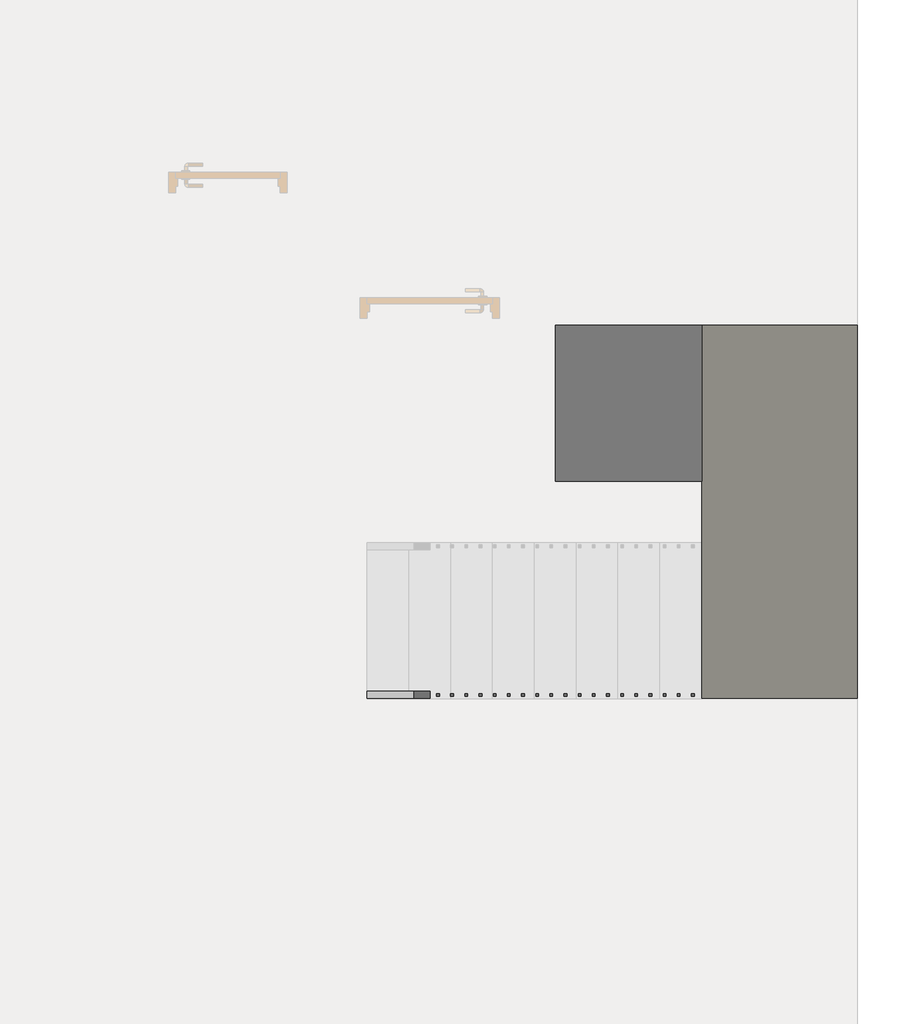
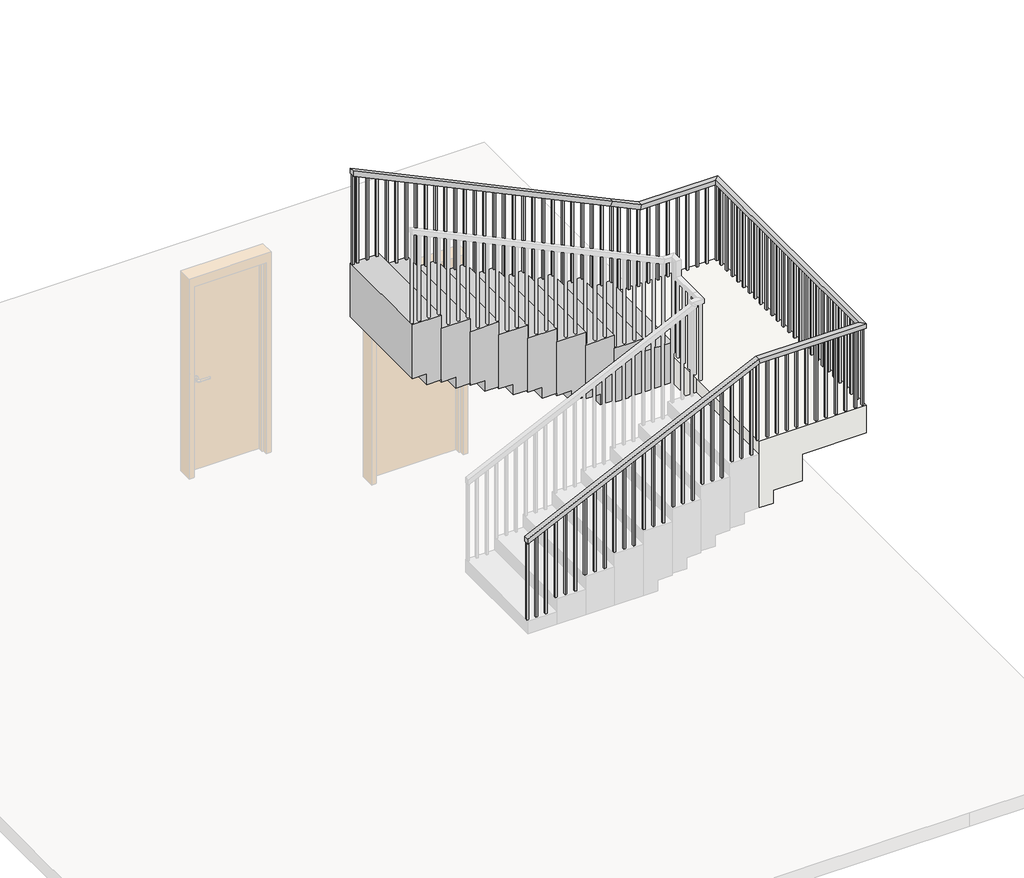
# One storey, part 2 of 2: 1 railing, 1 slab, 1 stair flight.
"""IFC4 building model written with IfcOpenShell, lengths in millimetres."""

from ifc_helpers import new_model, si_unit, frame, origin, place, context, project, spatial, polyline, outline, extrude, faceted_brep, element, save

model = new_model("IFC4")

# Units and contexts
model_context = context("Model", 3, world=origin())
ifc_project = project(units=[si_unit("LENGTHUNIT", "METRE", prefix="MILLI")], contexts=[model_context])

# Site, building, storey
site = spatial("IfcSite", under=ifc_project)
building = spatial("IfcBuilding", under=site)
storey = spatial("IfcBuildingStorey", under=building, Elevation=600.0)

# Railing
placement = place(None, origin())
element("IfcRailing", 1, ObjectType="Handrail - Rectangular", at=placement, inside=storey, context=model_context, shape_type="SolidModel", body=[
    faceted_brep([(-11513.3520625, -4858.6480844, 1642.1052632), (-11513.3520625, -4858.6480844, 1586.7794841), (-11513.3520625, -4908.6480844, 1586.7794841), (-11513.3520625, -4908.6480844, 1642.1052632), (-9113.3520625, -4858.6480844, 2778.9473684), (-9102.1087512, -4858.6480844, 2728.9473684), (-9102.1087512, -4908.6480844, 2728.9473684), (-9113.3520625, -4908.6480844, 2778.9473684), (-8046.1520625, -4858.6480844, 2778.9473684), (-8046.1520625, -4858.6480844, 2728.9473684), (-7996.1520625, -4908.6480844, 2728.9473684), (-7996.1520625, -4908.6480844, 2778.9473684), (-8046.1520625, -2284.4480844, 2778.9473684), (-8046.1520625, -2284.4480844, 2728.9473684), (-7996.1520625, -2234.4480844, 2728.9473684), (-7996.1520625, -2234.4480844, 2778.9473684), (-8813.3520625, -2284.4480844, 2778.9473684), (-8824.5953738, -2284.4480844, 2728.9473684), (-8824.5953738, -2234.4480844, 2728.9473684), (-8813.3520625, -2234.4480844, 2778.9473684), (-9113.3520625, -2284.4480844, 2921.0526316), (-9134.7563797, -2284.4480844, 2875.8657396), (-9134.7563797, -2234.4480844, 2875.8657396), (-9113.3520625, -2234.4480844, 2921.0526316), (-11813.3520625, -2284.4480844, 4200.0), (-11813.3520625, -2234.4480844, 4200.0), (-11813.3520625, -2234.4480844, 4144.6742209), (-11813.3520625, -2284.4480844, 4144.6742209)], [[[0, 1, 2, 3]], [[1, 0, 4, 5]], [[2, 1, 5, 6]], [[3, 2, 6, 7]], [[0, 3, 7, 4]], [[5, 4, 8, 9]], [[6, 5, 9, 10]], [[7, 6, 10, 11]], [[4, 7, 11, 8]], [[9, 8, 12, 13]], [[10, 9, 13, 14]], [[11, 10, 14, 15]], [[8, 11, 15, 12]], [[13, 12, 16, 17]], [[14, 13, 17, 18]], [[15, 14, 18, 19]], [[12, 15, 19, 16]], [[17, 16, 20, 21]], [[18, 17, 21, 22]], [[19, 18, 22, 23]], [[16, 19, 23, 20]], [[24, 25, 26, 27]], [[21, 20, 24, 27]], [[22, 21, 27, 26]], [[23, 22, 26, 25]], [[20, 23, 25, 24]]]),
    extrude(outline(polyline([(3157.8947368, -11744.9520625), (4112.2742209, -11744.9520625), (4121.7479052, -11764.9520625), (3157.8947368, -11764.9520625), (3157.8947368, -11744.9520625)])), frame((0.0, -2269.4480844, 0.0), z_axis=(0.0, 1.0, 0.0), x_axis=(0.0, 0.0, 1.0)), (0.0, 0.0, 1.0), 20.0),
    extrude(outline(polyline([(3157.8947368, -11643.3520625), (4064.1479052, -11643.3520625), (4073.6215894, -11663.3520625), (3157.8947368, -11663.3520625), (3157.8947368, -11643.3520625)])), frame((0.0, -2269.4480844, 0.0), z_axis=(0.0, 1.0, 0.0), x_axis=(0.0, 0.0, 1.0)), (0.0, 0.0, 1.0), 20.0),
    extrude(outline(polyline([(3157.8947368, -11541.7520625), (4016.0215894, -11541.7520625), (4025.4952736, -11561.7520625), (3157.8947368, -11561.7520625), (3157.8947368, -11541.7520625)])), frame((0.0, -2269.4480844, 0.0), z_axis=(0.0, 1.0, 0.0), x_axis=(0.0, 0.0, 1.0)), (0.0, 0.0, 1.0), 20.0),
    extrude(outline(polyline([(3015.7894737, -11440.1520625), (3967.8952736, -11440.1520625), (3977.3689578, -11460.1520625), (3015.7894737, -11460.1520625), (3015.7894737, -11440.1520625)])), frame((0.0, -2269.4480844, 0.0), z_axis=(0.0, 1.0, 0.0), x_axis=(0.0, 0.0, 1.0)), (0.0, 0.0, 1.0), 20.0),
    extrude(outline(polyline([(3015.7894737, -11338.5520625), (3919.7689578, -11338.5520625), (3929.242642, -11358.5520625), (3015.7894737, -11358.5520625), (3015.7894737, -11338.5520625)])), frame((0.0, -2269.4480844, 0.0), z_axis=(0.0, 1.0, 0.0), x_axis=(0.0, 0.0, 1.0)), (0.0, 0.0, 1.0), 20.0),
    extrude(outline(polyline([(3015.7894737, -11236.9520625), (3871.642642, -11236.9520625), (3881.1163262, -11256.9520625), (3015.7894737, -11256.9520625), (3015.7894737, -11236.9520625)])), frame((0.0, -2269.4480844, 0.0), z_axis=(0.0, 1.0, 0.0), x_axis=(0.0, 0.0, 1.0)), (0.0, 0.0, 1.0), 20.0),
    extrude(outline(polyline([(2873.6842105, -11135.3520625), (3823.5163262, -11135.3520625), (3832.9900104, -11155.3520625), (2873.6842105, -11155.3520625), (2873.6842105, -11135.3520625)])), frame((0.0, -2269.4480844, 0.0), z_axis=(0.0, 1.0, 0.0), x_axis=(0.0, 0.0, 1.0)), (0.0, 0.0, 1.0), 20.0),
    extrude(outline(polyline([(2873.6842105, -11033.7520625), (3775.3900104, -11033.7520625), (3784.8636946, -11053.7520625), (2873.6842105, -11053.7520625), (2873.6842105, -11033.7520625)])), frame((0.0, -2269.4480844, 0.0), z_axis=(0.0, 1.0, 0.0), x_axis=(0.0, 0.0, 1.0)), (0.0, 0.0, 1.0), 20.0),
    extrude(outline(polyline([(2873.6842105, -10932.1520625), (3727.2636946, -10932.1520625), (3736.7373788, -10952.1520625), (2873.6842105, -10952.1520625), (2873.6842105, -10932.1520625)])), frame((0.0, -2269.4480844, 0.0), z_axis=(0.0, 1.0, 0.0), x_axis=(0.0, 0.0, 1.0)), (0.0, 0.0, 1.0), 20.0),
    extrude(outline(polyline([(2731.5789474, -10830.5520625), (3679.1373788, -10830.5520625), (3688.611063, -10850.5520625), (2731.5789474, -10850.5520625), (2731.5789474, -10830.5520625)])), frame((0.0, -2269.4480844, 0.0), z_axis=(0.0, 1.0, 0.0), x_axis=(0.0, 0.0, 1.0)), (0.0, 0.0, 1.0), 20.0),
    extrude(outline(polyline([(2731.5789474, -10728.9520625), (3631.011063, -10728.9520625), (3640.4847473, -10748.9520625), (2731.5789474, -10748.9520625), (2731.5789474, -10728.9520625)])), frame((0.0, -2269.4480844, 0.0), z_axis=(0.0, 1.0, 0.0), x_axis=(0.0, 0.0, 1.0)), (0.0, 0.0, 1.0), 20.0),
    extrude(outline(polyline([(2731.5789474, -10627.3520625), (3582.8847473, -10627.3520625), (3592.3584315, -10647.3520625), (2731.5789474, -10647.3520625), (2731.5789474, -10627.3520625)])), frame((0.0, -2269.4480844, 0.0), z_axis=(0.0, 1.0, 0.0), x_axis=(0.0, 0.0, 1.0)), (0.0, 0.0, 1.0), 20.0),
    extrude(outline(polyline([(2589.4736842, -10525.7520625), (3534.7584315, -10525.7520625), (3544.2321157, -10545.7520625), (2589.4736842, -10545.7520625), (2589.4736842, -10525.7520625)])), frame((0.0, -2269.4480844, 0.0), z_axis=(0.0, 1.0, 0.0), x_axis=(0.0, 0.0, 1.0)), (0.0, 0.0, 1.0), 20.0),
    extrude(outline(polyline([(2589.4736842, -10424.1520625), (3486.6321157, -10424.1520625), (3496.1057999, -10444.1520625), (2589.4736842, -10444.1520625), (2589.4736842, -10424.1520625)])), frame((0.0, -2269.4480844, 0.0), z_axis=(0.0, 1.0, 0.0), x_axis=(0.0, 0.0, 1.0)), (0.0, 0.0, 1.0), 20.0),
    extrude(outline(polyline([(2589.4736842, -10322.5520625), (3438.5057999, -10322.5520625), (3447.9794841, -10342.5520625), (2589.4736842, -10342.5520625), (2589.4736842, -10322.5520625)])), frame((0.0, -2269.4480844, 0.0), z_axis=(0.0, 1.0, 0.0), x_axis=(0.0, 0.0, 1.0)), (0.0, 0.0, 1.0), 20.0),
    extrude(outline(polyline([(2447.3684211, -10220.9520625), (3390.3794841, -10220.9520625), (3399.8531683, -10240.9520625), (2447.3684211, -10240.9520625), (2447.3684211, -10220.9520625)])), frame((0.0, -2269.4480844, 0.0), z_axis=(0.0, 1.0, 0.0), x_axis=(0.0, 0.0, 1.0)), (0.0, 0.0, 1.0), 20.0),
    extrude(outline(polyline([(2447.3684211, -10119.3520625), (3342.2531683, -10119.3520625), (3351.7268525, -10139.3520625), (2447.3684211, -10139.3520625), (2447.3684211, -10119.3520625)])), frame((0.0, -2269.4480844, 0.0), z_axis=(0.0, 1.0, 0.0), x_axis=(0.0, 0.0, 1.0)), (0.0, 0.0, 1.0), 20.0),
    extrude(outline(polyline([(2447.3684211, -10017.7520625), (3294.1268525, -10017.7520625), (3303.6005367, -10037.7520625), (2447.3684211, -10037.7520625), (2447.3684211, -10017.7520625)])), frame((0.0, -2269.4480844, 0.0), z_axis=(0.0, 1.0, 0.0), x_axis=(0.0, 0.0, 1.0)), (0.0, 0.0, 1.0), 20.0),
    extrude(outline(polyline([(2305.2631579, -9916.1520625), (3246.0005367, -9916.1520625), (3255.4742209, -9936.1520625), (2305.2631579, -9936.1520625), (2305.2631579, -9916.1520625)])), frame((0.0, -2269.4480844, 0.0), z_axis=(0.0, 1.0, 0.0), x_axis=(0.0, 0.0, 1.0)), (0.0, 0.0, 1.0), 20.0),
    extrude(outline(polyline([(2305.2631579, -9814.5520625), (3197.8742209, -9814.5520625), (3207.3479052, -9834.5520625), (2305.2631579, -9834.5520625), (2305.2631579, -9814.5520625)])), frame((0.0, -2269.4480844, 0.0), z_axis=(0.0, 1.0, 0.0), x_axis=(0.0, 0.0, 1.0)), (0.0, 0.0, 1.0), 20.0),
    extrude(outline(polyline([(2305.2631579, -9712.9520625), (3149.7005367, -9712.9520625), (3159.1742209, -9732.9520625), (2305.2631579, -9732.9520625), (2305.2631579, -9712.9520625)])), frame((0.0, -2269.4480844, 0.0), z_axis=(0.0, 1.0, 0.0), x_axis=(0.0, 0.0, 1.0)), (0.0, 0.0, 1.0), 20.0),
    extrude(outline(polyline([(2163.1578947, -9611.3520625), (3101.6215894, -9611.3520625), (3111.0952736, -9631.3520625), (2163.1578947, -9631.3520625), (2163.1578947, -9611.3520625)])), frame((0.0, -2269.4480844, 0.0), z_axis=(0.0, 1.0, 0.0), x_axis=(0.0, 0.0, 1.0)), (0.0, 0.0, 1.0), 20.0),
    extrude(outline(polyline([(2163.1578947, -9509.7520625), (3053.4952736, -9509.7520625), (3062.9689578, -9529.7520625), (2163.1578947, -9529.7520625), (2163.1578947, -9509.7520625)])), frame((0.0, -2269.4480844, 0.0), z_axis=(0.0, 1.0, 0.0), x_axis=(0.0, 0.0, 1.0)), (0.0, 0.0, 1.0), 20.0),
    extrude(outline(polyline([(2163.1578947, -9408.1520625), (3005.3689578, -9408.1520625), (3014.842642, -9428.1520625), (2163.1578947, -9428.1520625), (2163.1578947, -9408.1520625)])), frame((0.0, -2269.4480844, 0.0), z_axis=(0.0, 1.0, 0.0), x_axis=(0.0, 0.0, 1.0)), (0.0, 0.0, 1.0), 20.0),
    extrude(outline(polyline([(2021.0526316, -9306.5520625), (2957.242642, -9306.5520625), (2966.7163262, -9326.5520625), (2021.0526316, -9326.5520625), (2021.0526316, -9306.5520625)])), frame((0.0, -2269.4480844, 0.0), z_axis=(0.0, 1.0, 0.0), x_axis=(0.0, 0.0, 1.0)), (0.0, 0.0, 1.0), 20.0),
    extrude(outline(polyline([(2021.0526316, -9204.9520625), (2909.1163262, -9204.9520625), (2918.5900104, -9224.9520625), (2021.0526316, -9224.9520625), (2021.0526316, -9204.9520625)])), frame((0.0, -2269.4480844, 0.0), z_axis=(0.0, 1.0, 0.0), x_axis=(0.0, 0.0, 1.0)), (0.0, 0.0, 1.0), 20.0),
    extrude(outline(polyline([(1878.9473684, -9027.1520625), (2824.8952736, -9027.1520625), (2834.3689578, -9047.1520625), (1878.9473684, -9047.1520625), (1878.9473684, -9027.1520625)])), frame((0.0, -2269.4480844, 0.0), z_axis=(0.0, 1.0, 0.0), x_axis=(0.0, 0.0, 1.0)), (0.0, 0.0, 1.0), 20.0),
    extrude(outline(polyline([(1878.9473684, -8925.5520625), (2776.7689578, -8925.5520625), (2786.242642, -8945.5520625), (1878.9473684, -8945.5520625), (1878.9473684, -8925.5520625)])), frame((0.0, -2269.4480844, 0.0), z_axis=(0.0, 1.0, 0.0), x_axis=(0.0, 0.0, 1.0)), (0.0, 0.0, 1.0), 20.0),
    extrude(outline(polyline([(1878.9473684, -8823.9520625), (2728.642642, -8823.9520625), (2738.1163262, -8843.9520625), (1878.9473684, -8843.9520625), (1878.9473684, -8823.9520625)])), frame((0.0, -2269.4480844, 0.0), z_axis=(0.0, 1.0, 0.0), x_axis=(0.0, 0.0, 1.0)), (0.0, 0.0, 1.0), 20.0),
    extrude(outline(polyline([(-8722.3520625, -2249.4480844), (-8722.3520625, -2269.4480844), (-8742.3520625, -2269.4480844), (-8742.3520625, -2249.4480844), (-8722.3520625, -2249.4480844)])), frame((0.0, 0.0, 1878.9473684), z_axis=(0.0, 0.0, 1.0), x_axis=(1.0, 0.0, 0.0)), (0.0, 0.0, 1.0), 850.0),
    extrude(outline(polyline([(-8620.7520625, -2249.4480844), (-8620.7520625, -2269.4480844), (-8640.7520625, -2269.4480844), (-8640.7520625, -2249.4480844), (-8620.7520625, -2249.4480844)])), frame((0.0, 0.0, 1878.9473684), z_axis=(0.0, 0.0, 1.0), x_axis=(1.0, 0.0, 0.0)), (0.0, 0.0, 1.0), 850.0),
    extrude(outline(polyline([(-8519.1520625, -2249.4480844), (-8519.1520625, -2269.4480844), (-8539.1520625, -2269.4480844), (-8539.1520625, -2249.4480844), (-8519.1520625, -2249.4480844)])), frame((0.0, 0.0, 1878.9473684), z_axis=(0.0, 0.0, 1.0), x_axis=(1.0, 0.0, 0.0)), (0.0, 0.0, 1.0), 850.0),
    extrude(outline(polyline([(-8417.5520625, -2249.4480844), (-8417.5520625, -2269.4480844), (-8437.5520625, -2269.4480844), (-8437.5520625, -2249.4480844), (-8417.5520625, -2249.4480844)])), frame((0.0, 0.0, 1878.9473684), z_axis=(0.0, 0.0, 1.0), x_axis=(1.0, 0.0, 0.0)), (0.0, 0.0, 1.0), 850.0),
    extrude(outline(polyline([(-8315.9520625, -2249.4480844), (-8315.9520625, -2269.4480844), (-8335.9520625, -2269.4480844), (-8335.9520625, -2249.4480844), (-8315.9520625, -2249.4480844)])), frame((0.0, 0.0, 1878.9473684), z_axis=(0.0, 0.0, 1.0), x_axis=(1.0, 0.0, 0.0)), (0.0, 0.0, 1.0), 850.0),
    extrude(outline(polyline([(-8214.3520625, -2249.4480844), (-8214.3520625, -2269.4480844), (-8234.3520625, -2269.4480844), (-8234.3520625, -2249.4480844), (-8214.3520625, -2249.4480844)])), frame((0.0, 0.0, 1878.9473684), z_axis=(0.0, 0.0, 1.0), x_axis=(1.0, 0.0, 0.0)), (0.0, 0.0, 1.0), 850.0),
    extrude(outline(polyline([(-8112.7520625, -2249.4480844), (-8112.7520625, -2269.4480844), (-8132.7520625, -2269.4480844), (-8132.7520625, -2249.4480844), (-8112.7520625, -2249.4480844)])), frame((0.0, 0.0, 1878.9473684), z_axis=(0.0, 0.0, 1.0), x_axis=(1.0, 0.0, 0.0)), (0.0, 0.0, 1.0), 850.0),
    extrude(outline(polyline([(-8011.1520625, -2353.6480844), (-8031.1520625, -2353.6480844), (-8031.1520625, -2333.6480844), (-8011.1520625, -2333.6480844), (-8011.1520625, -2353.6480844)])), frame((0.0, 0.0, 1878.9473684), z_axis=(0.0, 0.0, 1.0), x_axis=(1.0, 0.0, 0.0)), (0.0, 0.0, 1.0), 850.0),
    extrude(outline(polyline([(-8011.1520625, -2455.2480844), (-8031.1520625, -2455.2480844), (-8031.1520625, -2435.2480844), (-8011.1520625, -2435.2480844), (-8011.1520625, -2455.2480844)])), frame((0.0, 0.0, 1878.9473684), z_axis=(0.0, 0.0, 1.0), x_axis=(1.0, 0.0, 0.0)), (0.0, 0.0, 1.0), 850.0),
    extrude(outline(polyline([(-8011.1520625, -2556.8480844), (-8031.1520625, -2556.8480844), (-8031.1520625, -2536.8480844), (-8011.1520625, -2536.8480844), (-8011.1520625, -2556.8480844)])), frame((0.0, 0.0, 1878.9473684), z_axis=(0.0, 0.0, 1.0), x_axis=(1.0, 0.0, 0.0)), (0.0, 0.0, 1.0), 850.0),
    extrude(outline(polyline([(-8011.1520625, -2658.4480844), (-8031.1520625, -2658.4480844), (-8031.1520625, -2638.4480844), (-8011.1520625, -2638.4480844), (-8011.1520625, -2658.4480844)])), frame((0.0, 0.0, 1878.9473684), z_axis=(0.0, 0.0, 1.0), x_axis=(1.0, 0.0, 0.0)), (0.0, 0.0, 1.0), 850.0),
    extrude(outline(polyline([(-8011.1520625, -2760.0480844), (-8031.1520625, -2760.0480844), (-8031.1520625, -2740.0480844), (-8011.1520625, -2740.0480844), (-8011.1520625, -2760.0480844)])), frame((0.0, 0.0, 1878.9473684), z_axis=(0.0, 0.0, 1.0), x_axis=(1.0, 0.0, 0.0)), (0.0, 0.0, 1.0), 850.0),
    extrude(outline(polyline([(-8011.1520625, -2861.6480844), (-8031.1520625, -2861.6480844), (-8031.1520625, -2841.6480844), (-8011.1520625, -2841.6480844), (-8011.1520625, -2861.6480844)])), frame((0.0, 0.0, 1878.9473684), z_axis=(0.0, 0.0, 1.0), x_axis=(1.0, 0.0, 0.0)), (0.0, 0.0, 1.0), 850.0),
    extrude(outline(polyline([(-8011.1520625, -2963.2480844), (-8031.1520625, -2963.2480844), (-8031.1520625, -2943.2480844), (-8011.1520625, -2943.2480844), (-8011.1520625, -2963.2480844)])), frame((0.0, 0.0, 1878.9473684), z_axis=(0.0, 0.0, 1.0), x_axis=(1.0, 0.0, 0.0)), (0.0, 0.0, 1.0), 850.0),
    extrude(outline(polyline([(-8011.1520625, -3064.8480844), (-8031.1520625, -3064.8480844), (-8031.1520625, -3044.8480844), (-8011.1520625, -3044.8480844), (-8011.1520625, -3064.8480844)])), frame((0.0, 0.0, 1878.9473684), z_axis=(0.0, 0.0, 1.0), x_axis=(1.0, 0.0, 0.0)), (0.0, 0.0, 1.0), 850.0),
    extrude(outline(polyline([(-8011.1520625, -3166.4480844), (-8031.1520625, -3166.4480844), (-8031.1520625, -3146.4480844), (-8011.1520625, -3146.4480844), (-8011.1520625, -3166.4480844)])), frame((0.0, 0.0, 1878.9473684), z_axis=(0.0, 0.0, 1.0), x_axis=(1.0, 0.0, 0.0)), (0.0, 0.0, 1.0), 850.0),
    extrude(outline(polyline([(-8011.1520625, -3268.0480844), (-8031.1520625, -3268.0480844), (-8031.1520625, -3248.0480844), (-8011.1520625, -3248.0480844), (-8011.1520625, -3268.0480844)])), frame((0.0, 0.0, 1878.9473684), z_axis=(0.0, 0.0, 1.0), x_axis=(1.0, 0.0, 0.0)), (0.0, 0.0, 1.0), 850.0),
    extrude(outline(polyline([(-8011.1520625, -3369.6480844), (-8031.1520625, -3369.6480844), (-8031.1520625, -3349.6480844), (-8011.1520625, -3349.6480844), (-8011.1520625, -3369.6480844)])), frame((0.0, 0.0, 1878.9473684), z_axis=(0.0, 0.0, 1.0), x_axis=(1.0, 0.0, 0.0)), (0.0, 0.0, 1.0), 850.0),
    extrude(outline(polyline([(-8011.1520625, -3471.2480844), (-8031.1520625, -3471.2480844), (-8031.1520625, -3451.2480844), (-8011.1520625, -3451.2480844), (-8011.1520625, -3471.2480844)])), frame((0.0, 0.0, 1878.9473684), z_axis=(0.0, 0.0, 1.0), x_axis=(1.0, 0.0, 0.0)), (0.0, 0.0, 1.0), 850.0),
    extrude(outline(polyline([(-8011.1520625, -3572.8480844), (-8031.1520625, -3572.8480844), (-8031.1520625, -3552.8480844), (-8011.1520625, -3552.8480844), (-8011.1520625, -3572.8480844)])), frame((0.0, 0.0, 1878.9473684), z_axis=(0.0, 0.0, 1.0), x_axis=(1.0, 0.0, 0.0)), (0.0, 0.0, 1.0), 850.0),
    extrude(outline(polyline([(-8011.1520625, -3674.4480844), (-8031.1520625, -3674.4480844), (-8031.1520625, -3654.4480844), (-8011.1520625, -3654.4480844), (-8011.1520625, -3674.4480844)])), frame((0.0, 0.0, 1878.9473684), z_axis=(0.0, 0.0, 1.0), x_axis=(1.0, 0.0, 0.0)), (0.0, 0.0, 1.0), 850.0),
    extrude(outline(polyline([(-8011.1520625, -3776.0480844), (-8031.1520625, -3776.0480844), (-8031.1520625, -3756.0480844), (-8011.1520625, -3756.0480844), (-8011.1520625, -3776.0480844)])), frame((0.0, 0.0, 1878.9473684), z_axis=(0.0, 0.0, 1.0), x_axis=(1.0, 0.0, 0.0)), (0.0, 0.0, 1.0), 850.0),
    extrude(outline(polyline([(-8011.1520625, -3877.6480844), (-8031.1520625, -3877.6480844), (-8031.1520625, -3857.6480844), (-8011.1520625, -3857.6480844), (-8011.1520625, -3877.6480844)])), frame((0.0, 0.0, 1878.9473684), z_axis=(0.0, 0.0, 1.0), x_axis=(1.0, 0.0, 0.0)), (0.0, 0.0, 1.0), 850.0),
    extrude(outline(polyline([(-8011.1520625, -3979.2480844), (-8031.1520625, -3979.2480844), (-8031.1520625, -3959.2480844), (-8011.1520625, -3959.2480844), (-8011.1520625, -3979.2480844)])), frame((0.0, 0.0, 1878.9473684), z_axis=(0.0, 0.0, 1.0), x_axis=(1.0, 0.0, 0.0)), (0.0, 0.0, 1.0), 850.0),
    extrude(outline(polyline([(-8011.1520625, -4080.8480844), (-8031.1520625, -4080.8480844), (-8031.1520625, -4060.8480844), (-8011.1520625, -4060.8480844), (-8011.1520625, -4080.8480844)])), frame((0.0, 0.0, 1878.9473684), z_axis=(0.0, 0.0, 1.0), x_axis=(1.0, 0.0, 0.0)), (0.0, 0.0, 1.0), 850.0),
    extrude(outline(polyline([(-8011.1520625, -4182.4480844), (-8031.1520625, -4182.4480844), (-8031.1520625, -4162.4480844), (-8011.1520625, -4162.4480844), (-8011.1520625, -4182.4480844)])), frame((0.0, 0.0, 1878.9473684), z_axis=(0.0, 0.0, 1.0), x_axis=(1.0, 0.0, 0.0)), (0.0, 0.0, 1.0), 850.0),
    extrude(outline(polyline([(-8011.1520625, -4284.0480844), (-8031.1520625, -4284.0480844), (-8031.1520625, -4264.0480844), (-8011.1520625, -4264.0480844), (-8011.1520625, -4284.0480844)])), frame((0.0, 0.0, 1878.9473684), z_axis=(0.0, 0.0, 1.0), x_axis=(1.0, 0.0, 0.0)), (0.0, 0.0, 1.0), 850.0),
    extrude(outline(polyline([(-8011.1520625, -4385.6480844), (-8031.1520625, -4385.6480844), (-8031.1520625, -4365.6480844), (-8011.1520625, -4365.6480844), (-8011.1520625, -4385.6480844)])), frame((0.0, 0.0, 1878.9473684), z_axis=(0.0, 0.0, 1.0), x_axis=(1.0, 0.0, 0.0)), (0.0, 0.0, 1.0), 850.0),
    extrude(outline(polyline([(-8011.1520625, -4487.2480844), (-8031.1520625, -4487.2480844), (-8031.1520625, -4467.2480844), (-8011.1520625, -4467.2480844), (-8011.1520625, -4487.2480844)])), frame((0.0, 0.0, 1878.9473684), z_axis=(0.0, 0.0, 1.0), x_axis=(1.0, 0.0, 0.0)), (0.0, 0.0, 1.0), 850.0),
    extrude(outline(polyline([(-8011.1520625, -4588.8480844), (-8031.1520625, -4588.8480844), (-8031.1520625, -4568.8480844), (-8011.1520625, -4568.8480844), (-8011.1520625, -4588.8480844)])), frame((0.0, 0.0, 1878.9473684), z_axis=(0.0, 0.0, 1.0), x_axis=(1.0, 0.0, 0.0)), (0.0, 0.0, 1.0), 850.0),
    extrude(outline(polyline([(-8011.1520625, -4690.4480844), (-8031.1520625, -4690.4480844), (-8031.1520625, -4670.4480844), (-8011.1520625, -4670.4480844), (-8011.1520625, -4690.4480844)])), frame((0.0, 0.0, 1878.9473684), z_axis=(0.0, 0.0, 1.0), x_axis=(1.0, 0.0, 0.0)), (0.0, 0.0, 1.0), 850.0),
    extrude(outline(polyline([(-8011.1520625, -4792.0480844), (-8031.1520625, -4792.0480844), (-8031.1520625, -4772.0480844), (-8011.1520625, -4772.0480844), (-8011.1520625, -4792.0480844)])), frame((0.0, 0.0, 1878.9473684), z_axis=(0.0, 0.0, 1.0), x_axis=(1.0, 0.0, 0.0)), (0.0, 0.0, 1.0), 850.0),
    extrude(outline(polyline([(-8107.3520625, -4893.6480844), (-8107.3520625, -4873.6480844), (-8087.3520625, -4873.6480844), (-8087.3520625, -4893.6480844), (-8107.3520625, -4893.6480844)])), frame((0.0, 0.0, 1878.9473684), z_axis=(0.0, 0.0, 1.0), x_axis=(1.0, 0.0, 0.0)), (0.0, 0.0, 1.0), 850.0),
    extrude(outline(polyline([(-8208.9520625, -4893.6480844), (-8208.9520625, -4873.6480844), (-8188.9520625, -4873.6480844), (-8188.9520625, -4893.6480844), (-8208.9520625, -4893.6480844)])), frame((0.0, 0.0, 1878.9473684), z_axis=(0.0, 0.0, 1.0), x_axis=(1.0, 0.0, 0.0)), (0.0, 0.0, 1.0), 850.0),
    extrude(outline(polyline([(-8310.5520625, -4893.6480844), (-8310.5520625, -4873.6480844), (-8290.5520625, -4873.6480844), (-8290.5520625, -4893.6480844), (-8310.5520625, -4893.6480844)])), frame((0.0, 0.0, 1878.9473684), z_axis=(0.0, 0.0, 1.0), x_axis=(1.0, 0.0, 0.0)), (0.0, 0.0, 1.0), 850.0),
    extrude(outline(polyline([(-8412.1520625, -4893.6480844), (-8412.1520625, -4873.6480844), (-8392.1520625, -4873.6480844), (-8392.1520625, -4893.6480844), (-8412.1520625, -4893.6480844)])), frame((0.0, 0.0, 1878.9473684), z_axis=(0.0, 0.0, 1.0), x_axis=(1.0, 0.0, 0.0)), (0.0, 0.0, 1.0), 850.0),
    extrude(outline(polyline([(-8513.7520625, -4893.6480844), (-8513.7520625, -4873.6480844), (-8493.7520625, -4873.6480844), (-8493.7520625, -4893.6480844), (-8513.7520625, -4893.6480844)])), frame((0.0, 0.0, 1878.9473684), z_axis=(0.0, 0.0, 1.0), x_axis=(1.0, 0.0, 0.0)), (0.0, 0.0, 1.0), 850.0),
    extrude(outline(polyline([(-8615.3520625, -4893.6480844), (-8615.3520625, -4873.6480844), (-8595.3520625, -4873.6480844), (-8595.3520625, -4893.6480844), (-8615.3520625, -4893.6480844)])), frame((0.0, 0.0, 1878.9473684), z_axis=(0.0, 0.0, 1.0), x_axis=(1.0, 0.0, 0.0)), (0.0, 0.0, 1.0), 850.0),
    extrude(outline(polyline([(-8716.9520625, -4893.6480844), (-8716.9520625, -4873.6480844), (-8696.9520625, -4873.6480844), (-8696.9520625, -4893.6480844), (-8716.9520625, -4893.6480844)])), frame((0.0, 0.0, 1878.9473684), z_axis=(0.0, 0.0, 1.0), x_axis=(1.0, 0.0, 0.0)), (0.0, 0.0, 1.0), 850.0),
    extrude(outline(polyline([(-8818.5520625, -4893.6480844), (-8818.5520625, -4873.6480844), (-8798.5520625, -4873.6480844), (-8798.5520625, -4893.6480844), (-8818.5520625, -4893.6480844)])), frame((0.0, 0.0, 1878.9473684), z_axis=(0.0, 0.0, 1.0), x_axis=(1.0, 0.0, 0.0)), (0.0, 0.0, 1.0), 850.0),
    extrude(outline(polyline([(-8920.1520625, -4893.6480844), (-8920.1520625, -4873.6480844), (-8900.1520625, -4873.6480844), (-8900.1520625, -4893.6480844), (-8920.1520625, -4893.6480844)])), frame((0.0, 0.0, 1878.9473684), z_axis=(0.0, 0.0, 1.0), x_axis=(1.0, 0.0, 0.0)), (0.0, 0.0, 1.0), 850.0),
    extrude(outline(polyline([(-9021.7520625, -4893.6480844), (-9021.7520625, -4873.6480844), (-9001.7520625, -4873.6480844), (-9001.7520625, -4893.6480844), (-9021.7520625, -4893.6480844)])), frame((0.0, 0.0, 1878.9473684), z_axis=(0.0, 0.0, 1.0), x_axis=(1.0, 0.0, 0.0)), (0.0, 0.0, 1.0), 850.0),
    extrude(outline(polyline([(2688.9479052, -9186.5520625), (1736.8421053, -9186.5520625), (1736.8421053, -9166.5520625), (2698.4215894, -9166.5520625), (2688.9479052, -9186.5520625)])), frame((0.0, -4893.6480844, 0.0), z_axis=(0.0, 1.0, 0.0), x_axis=(0.0, 0.0, 1.0)), (0.0, 0.0, 1.0), 20.0),
    extrude(outline(polyline([(2640.8215894, -9288.1520625), (1736.8421053, -9288.1520625), (1736.8421053, -9268.1520625), (2650.2952736, -9268.1520625), (2640.8215894, -9288.1520625)])), frame((0.0, -4893.6480844, 0.0), z_axis=(0.0, 1.0, 0.0), x_axis=(0.0, 0.0, 1.0)), (0.0, 0.0, 1.0), 20.0),
    extrude(outline(polyline([(2592.6952736, -9389.7520625), (1736.8421053, -9389.7520625), (1736.8421053, -9369.7520625), (2602.1689578, -9369.7520625), (2592.6952736, -9389.7520625)])), frame((0.0, -4893.6480844, 0.0), z_axis=(0.0, 1.0, 0.0), x_axis=(0.0, 0.0, 1.0)), (0.0, 0.0, 1.0), 20.0),
    extrude(outline(polyline([(2544.5689578, -9491.3520625), (1594.7368421, -9491.3520625), (1594.7368421, -9471.3520625), (2554.042642, -9471.3520625), (2544.5689578, -9491.3520625)])), frame((0.0, -4893.6480844, 0.0), z_axis=(0.0, 1.0, 0.0), x_axis=(0.0, 0.0, 1.0)), (0.0, 0.0, 1.0), 20.0),
    extrude(outline(polyline([(2496.442642, -9592.9520625), (1594.7368421, -9592.9520625), (1594.7368421, -9572.9520625), (2505.9163262, -9572.9520625), (2496.442642, -9592.9520625)])), frame((0.0, -4893.6480844, 0.0), z_axis=(0.0, 1.0, 0.0), x_axis=(0.0, 0.0, 1.0)), (0.0, 0.0, 1.0), 20.0),
    extrude(outline(polyline([(2448.3163262, -9694.5520625), (1594.7368421, -9694.5520625), (1594.7368421, -9674.5520625), (2457.7900104, -9674.5520625), (2448.3163262, -9694.5520625)])), frame((0.0, -4893.6480844, 0.0), z_axis=(0.0, 1.0, 0.0), x_axis=(0.0, 0.0, 1.0)), (0.0, 0.0, 1.0), 20.0),
    extrude(outline(polyline([(2400.1900104, -9796.1520625), (1452.6315789, -9796.1520625), (1452.6315789, -9776.1520625), (2409.6636946, -9776.1520625), (2400.1900104, -9796.1520625)])), frame((0.0, -4893.6480844, 0.0), z_axis=(0.0, 1.0, 0.0), x_axis=(0.0, 0.0, 1.0)), (0.0, 0.0, 1.0), 20.0),
    extrude(outline(polyline([(2352.0636946, -9897.7520625), (1452.6315789, -9897.7520625), (1452.6315789, -9877.7520625), (2361.5373788, -9877.7520625), (2352.0636946, -9897.7520625)])), frame((0.0, -4893.6480844, 0.0), z_axis=(0.0, 1.0, 0.0), x_axis=(0.0, 0.0, 1.0)), (0.0, 0.0, 1.0), 20.0),
    extrude(outline(polyline([(2303.9373788, -9999.3520625), (1452.6315789, -9999.3520625), (1452.6315789, -9979.3520625), (2313.411063, -9979.3520625), (2303.9373788, -9999.3520625)])), frame((0.0, -4893.6480844, 0.0), z_axis=(0.0, 1.0, 0.0), x_axis=(0.0, 0.0, 1.0)), (0.0, 0.0, 1.0), 20.0),
    extrude(outline(polyline([(2255.811063, -10100.9520625), (1310.5263158, -10100.9520625), (1310.5263158, -10080.9520625), (2265.2847473, -10080.9520625), (2255.811063, -10100.9520625)])), frame((0.0, -4893.6480844, 0.0), z_axis=(0.0, 1.0, 0.0), x_axis=(0.0, 0.0, 1.0)), (0.0, 0.0, 1.0), 20.0),
    extrude(outline(polyline([(2207.6847473, -10202.5520625), (1310.5263158, -10202.5520625), (1310.5263158, -10182.5520625), (2217.1584315, -10182.5520625), (2207.6847473, -10202.5520625)])), frame((0.0, -4893.6480844, 0.0), z_axis=(0.0, 1.0, 0.0), x_axis=(0.0, 0.0, 1.0)), (0.0, 0.0, 1.0), 20.0),
    extrude(outline(polyline([(2159.5584315, -10304.1520625), (1310.5263158, -10304.1520625), (1310.5263158, -10284.1520625), (2169.0321157, -10284.1520625), (2159.5584315, -10304.1520625)])), frame((0.0, -4893.6480844, 0.0), z_axis=(0.0, 1.0, 0.0), x_axis=(0.0, 0.0, 1.0)), (0.0, 0.0, 1.0), 20.0),
    extrude(outline(polyline([(2111.4321157, -10405.7520625), (1168.4210526, -10405.7520625), (1168.4210526, -10385.7520625), (2120.9057999, -10385.7520625), (2111.4321157, -10405.7520625)])), frame((0.0, -4893.6480844, 0.0), z_axis=(0.0, 1.0, 0.0), x_axis=(0.0, 0.0, 1.0)), (0.0, 0.0, 1.0), 20.0),
    extrude(outline(polyline([(2063.3057999, -10507.3520625), (1168.4210526, -10507.3520625), (1168.4210526, -10487.3520625), (2072.7794841, -10487.3520625), (2063.3057999, -10507.3520625)])), frame((0.0, -4893.6480844, 0.0), z_axis=(0.0, 1.0, 0.0), x_axis=(0.0, 0.0, 1.0)), (0.0, 0.0, 1.0), 20.0),
    extrude(outline(polyline([(2015.1794841, -10608.9520625), (1168.4210526, -10608.9520625), (1168.4210526, -10588.9520625), (2024.6531683, -10588.9520625), (2015.1794841, -10608.9520625)])), frame((0.0, -4893.6480844, 0.0), z_axis=(0.0, 1.0, 0.0), x_axis=(0.0, 0.0, 1.0)), (0.0, 0.0, 1.0), 20.0),
    extrude(outline(polyline([(1967.0531683, -10710.5520625), (1026.3157895, -10710.5520625), (1026.3157895, -10690.5520625), (1976.5268525, -10690.5520625), (1967.0531683, -10710.5520625)])), frame((0.0, -4893.6480844, 0.0), z_axis=(0.0, 1.0, 0.0), x_axis=(0.0, 0.0, 1.0)), (0.0, 0.0, 1.0), 20.0),
    extrude(outline(polyline([(1918.9268525, -10812.1520625), (1026.3157895, -10812.1520625), (1026.3157895, -10792.1520625), (1928.4005367, -10792.1520625), (1918.9268525, -10812.1520625)])), frame((0.0, -4893.6480844, 0.0), z_axis=(0.0, 1.0, 0.0), x_axis=(0.0, 0.0, 1.0)), (0.0, 0.0, 1.0), 20.0),
    extrude(outline(polyline([(1870.7531683, -10913.7520625), (1026.3157895, -10913.7520625), (1026.3157895, -10893.7520625), (1880.2268525, -10893.7520625), (1870.7531683, -10913.7520625)])), frame((0.0, -4893.6480844, 0.0), z_axis=(0.0, 1.0, 0.0), x_axis=(0.0, 0.0, 1.0)), (0.0, 0.0, 1.0), 20.0),
    extrude(outline(polyline([(1822.6742209, -11015.3520625), (884.2105263, -11015.3520625), (884.2105263, -10995.3520625), (1832.1479052, -10995.3520625), (1822.6742209, -11015.3520625)])), frame((0.0, -4893.6480844, 0.0), z_axis=(0.0, 1.0, 0.0), x_axis=(0.0, 0.0, 1.0)), (0.0, 0.0, 1.0), 20.0),
    extrude(outline(polyline([(1774.5479052, -11116.9520625), (884.2105263, -11116.9520625), (884.2105263, -11096.9520625), (1784.0215894, -11096.9520625), (1774.5479052, -11116.9520625)])), frame((0.0, -4893.6480844, 0.0), z_axis=(0.0, 1.0, 0.0), x_axis=(0.0, 0.0, 1.0)), (0.0, 0.0, 1.0), 20.0),
    extrude(outline(polyline([(1726.4215894, -11218.5520625), (884.2105263, -11218.5520625), (884.2105263, -11198.5520625), (1735.8952736, -11198.5520625), (1726.4215894, -11218.5520625)])), frame((0.0, -4893.6480844, 0.0), z_axis=(0.0, 1.0, 0.0), x_axis=(0.0, 0.0, 1.0)), (0.0, 0.0, 1.0), 20.0),
    extrude(outline(polyline([(1678.2952736, -11320.1520625), (742.1052632, -11320.1520625), (742.1052632, -11300.1520625), (1687.7689578, -11300.1520625), (1678.2952736, -11320.1520625)])), frame((0.0, -4893.6480844, 0.0), z_axis=(0.0, 1.0, 0.0), x_axis=(0.0, 0.0, 1.0)), (0.0, 0.0, 1.0), 20.0),
    extrude(outline(polyline([(1630.1689578, -11421.7520625), (742.1052632, -11421.7520625), (742.1052632, -11401.7520625), (1639.642642, -11401.7520625), (1630.1689578, -11421.7520625)])), frame((0.0, -4893.6480844, 0.0), z_axis=(0.0, 1.0, 0.0), x_axis=(0.0, 0.0, 1.0)), (0.0, 0.0, 1.0), 20.0),
    extrude(outline(polyline([(1878.9473684, -9103.3520625), (2860.9900104, -9103.3520625), (2870.4636946, -9123.3520625), (1878.9473684, -9123.3520625), (1878.9473684, -9103.3520625)])), frame((0.0, -2269.4480844, 0.0), z_axis=(0.0, 1.0, 0.0), x_axis=(0.0, 0.0, 1.0)), (0.0, 0.0, 1.0), 20.0),
    extrude(outline(polyline([(-8011.1520625, -2269.4480844), (-8031.1520625, -2269.4480844), (-8031.1520625, -2249.4480844), (-8011.1520625, -2249.4480844), (-8011.1520625, -2269.4480844)])), frame((0.0, 0.0, 1878.9473684), z_axis=(0.0, 0.0, 1.0), x_axis=(1.0, 0.0, 0.0)), (0.0, 0.0, 1.0), 850.0),
    extrude(outline(polyline([(-8031.1520625, -4893.6480844), (-8031.1520625, -4873.6480844), (-8011.1520625, -4873.6480844), (-8011.1520625, -4893.6480844), (-8031.1520625, -4893.6480844)])), frame((0.0, 0.0, 1878.9473684), z_axis=(0.0, 0.0, 1.0), x_axis=(1.0, 0.0, 0.0)), (0.0, 0.0, 1.0), 850.0),
    extrude(outline(polyline([(2718.8847473, -9123.3520625), (1878.9473684, -9123.3520625), (1878.9473684, -9103.3520625), (2728.3584315, -9103.3520625), (2718.8847473, -9123.3520625)])), frame((0.0, -4893.6480844, 0.0), z_axis=(0.0, 1.0, 0.0), x_axis=(0.0, 0.0, 1.0)), (0.0, 0.0, 1.0), 20.0),
    extrude(outline(polyline([(3157.8947368, -11793.8520625), (4135.4373788, -11793.8520625), (4144.911063, -11813.8520625), (3157.8947368, -11813.8520625), (3157.8947368, -11793.8520625)])), frame((0.0, -2269.4480844, 0.0), z_axis=(0.0, 1.0, 0.0), x_axis=(0.0, 0.0, 1.0)), (0.0, 0.0, 1.0), 20.0),
    extrude(outline(polyline([(1586.542642, -11513.8520625), (742.1052632, -11513.8520625), (742.1052632, -11493.8520625), (1596.0163262, -11493.8520625), (1586.542642, -11513.8520625)])), frame((0.0, -4893.6480844, 0.0), z_axis=(0.0, 1.0, 0.0), x_axis=(0.0, 0.0, 1.0)), (0.0, 0.0, 1.0), 20.0),
])

# Slab
element("IfcSlab", 2, ObjectType="300 mm Thickness", at=placement, inside=storey, context=model_context, shape_type="Brep", body=[
    faceted_brep([(-9113.3520625, -3791.4480844, 1878.9473684), (-9113.3520625, -4909.0480844, 1878.9473684), (-8663.3520625, -4909.0480844, 1878.9473684), (-7995.7520625, -4909.0480844, 1878.9473684), (-7995.7520625, -2234.0480844, 1878.9473684), (-9113.3520625, -2234.0480844, 1878.9473684), (-9113.3520625, -3351.6480844, 1878.9473684), (-9113.3520625, -3791.4480844, 1578.9473684), (-9113.3520625, -3791.4480844, 1144.7368421), (-9113.3520625, -4909.0480844, 1144.7368421), (-9113.3520625, -4909.0480844, 1736.8421053), (-8963.3520625, -4909.0480844, 1144.7368421), (-8963.3520625, -4909.0480844, 1286.8421053), (-8663.3520625, -4909.0480844, 1286.8421053), (-8663.3520625, -4909.0480844, 1578.9473684), (-7995.7520625, -4909.0480844, 1578.9473684), (-7995.7520625, -2234.0480844, 1578.9473684), (-9113.3520625, -2234.0480844, 1578.9473684), (-9113.3520625, -3351.6480844, 1578.9473684), (-8663.3520625, -3791.4480844, 1578.9473684), (-8663.3520625, -3791.4480844, 1286.8421053), (-8963.3520625, -3791.4480844, 1286.8421053), (-8963.3520625, -3791.4480844, 1144.7368421)], [[[0, 1, 2, 3, 4, 5, 6]], [[1, 0, 7, 8, 9, 10]], [[1, 10, 9, 11, 12, 13, 14, 15, 3, 2]], [[4, 3, 15, 16]], [[5, 4, 16, 17]], [[6, 5, 17, 18]], [[0, 6, 18, 7]], [[19, 7, 18, 17, 16, 15, 14]], [[20, 21, 22, 8, 7, 19]], [[22, 11, 9, 8]], [[11, 22, 21, 12]], [[21, 20, 13, 12]], [[13, 20, 19, 14]]]),
])

# Stair flight
element("IfcStairFlight", 3, ObjectType="M_Monolithic Run", at=placement, inside=storey, context=model_context, shape_type="Brep", body=[
    faceted_brep([(-9413.3520625, -3351.6480844, 2021.0526316), (-9113.3520625, -3351.6480844, 2021.0526316), (-9113.3520625, -2234.0480844, 2021.0526316), (-9413.3520625, -2234.0480844, 2021.0526316), (-9413.3520625, -3351.6480844, 1578.9473684), (-9113.3520625, -3351.6480844, 1578.9473684), (-9113.3520625, -2234.0480844, 1578.9473684), (-9113.3520625, -2234.0480844, 1878.9473684), (-9413.3520625, -2234.0480844, 1578.9473684), (-9413.3520625, -3351.6480844, 2163.1578947), (-9413.3520625, -2234.0480844, 2163.1578947), (-9563.3520625, -2234.0480844, 2163.1578947), (-9713.3520625, -2234.0480844, 2163.1578947), (-9713.3520625, -3351.6480844, 2163.1578947), (-9563.3520625, -3351.6480844, 2163.1578947), (-9713.3520625, -3351.6480844, 1594.7368421), (-9713.3520625, -3351.6480844, 1571.0526316), (-9563.3520625, -3351.6480844, 1571.0526316), (-9563.3520625, -3351.6480844, 1578.9473684), (-9563.3520625, -2234.0480844, 1578.9473684), (-9563.3520625, -2234.0480844, 1571.0526316), (-9713.3520625, -2234.0480844, 1571.0526316), (-9713.3520625, -2234.0480844, 1594.7368421), (-10013.3520625, -3351.6480844, 2305.2631579), (-9713.3520625, -3351.6480844, 2305.2631579), (-9713.3520625, -2234.0480844, 2305.2631579), (-10013.3520625, -2234.0480844, 2305.2631579), (-9863.3520625, -3351.6480844, 1594.7368421), (-9863.3520625, -2234.0480844, 1594.7368421), (-10013.3520625, -3351.6480844, 1736.8421053), (-10013.3520625, -3351.6480844, 1713.1578947), (-9863.3520625, -3351.6480844, 1713.1578947), (-9863.3520625, -2234.0480844, 1713.1578947), (-10013.3520625, -2234.0480844, 1713.1578947), (-10013.3520625, -2234.0480844, 1736.8421053), (-10313.3520625, -3351.6480844, 2447.3684211), (-10013.3520625, -3351.6480844, 2447.3684211), (-10013.3520625, -2234.0480844, 2447.3684211), (-10313.3520625, -2234.0480844, 2447.3684211), (-10163.3520625, -3351.6480844, 1736.8421053), (-10163.3520625, -2234.0480844, 1736.8421053), (-10313.3520625, -3351.6480844, 1878.9473684), (-10313.3520625, -3351.6480844, 1855.2631579), (-10163.3520625, -3351.6480844, 1855.2631579), (-10163.3520625, -2234.0480844, 1855.2631579), (-10313.3520625, -2234.0480844, 1855.2631579), (-10313.3520625, -2234.0480844, 1878.9473684), (-10613.3520625, -3351.6480844, 2589.4736842), (-10313.3520625, -3351.6480844, 2589.4736842), (-10313.3520625, -2234.0480844, 2589.4736842), (-10613.3520625, -2234.0480844, 2589.4736842), (-10463.3520625, -3351.6480844, 1878.9473684), (-10463.3520625, -2234.0480844, 1878.9473684), (-10613.3520625, -3351.6480844, 2021.0526316), (-10613.3520625, -3351.6480844, 1997.3684211), (-10463.3520625, -3351.6480844, 1997.3684211), (-10463.3520625, -2234.0480844, 1997.3684211), (-10613.3520625, -2234.0480844, 1997.3684211), (-10613.3520625, -2234.0480844, 2021.0526316), (-10913.3520625, -3351.6480844, 2731.5789474), (-10613.3520625, -3351.6480844, 2731.5789474), (-10613.3520625, -2234.0480844, 2731.5789474), (-10913.3520625, -2234.0480844, 2731.5789474), (-10763.3520625, -3351.6480844, 2021.0526316), (-10763.3520625, -2234.0480844, 2021.0526316), (-10913.3520625, -3351.6480844, 2163.1578947), (-10913.3520625, -3351.6480844, 2139.4736842), (-10763.3520625, -3351.6480844, 2139.4736842), (-10763.3520625, -2234.0480844, 2139.4736842), (-10913.3520625, -2234.0480844, 2139.4736842), (-10913.3520625, -2234.0480844, 2163.1578947), (-11213.3520625, -3351.6480844, 2873.6842105), (-10913.3520625, -3351.6480844, 2873.6842105), (-10913.3520625, -2234.0480844, 2873.6842105), (-11213.3520625, -2234.0480844, 2873.6842105), (-11063.3520625, -3351.6480844, 2163.1578947), (-11063.3520625, -2234.0480844, 2163.1578947), (-11213.3520625, -3351.6480844, 2305.2631579), (-11213.3520625, -3351.6480844, 2281.5789474), (-11063.3520625, -3351.6480844, 2281.5789474), (-11063.3520625, -2234.0480844, 2281.5789474), (-11213.3520625, -2234.0480844, 2281.5789474), (-11213.3520625, -2234.0480844, 2305.2631579), (-11513.3520625, -3351.6480844, 3015.7894737), (-11213.3520625, -3351.6480844, 3015.7894737), (-11213.3520625, -2234.0480844, 3015.7894737), (-11513.3520625, -2234.0480844, 3015.7894737), (-11363.3520625, -3351.6480844, 2305.2631579), (-11363.3520625, -2234.0480844, 2305.2631579), (-11513.3520625, -3351.6480844, 2447.3684211), (-11513.3520625, -3351.6480844, 2423.6842105), (-11363.3520625, -3351.6480844, 2423.6842105), (-11363.3520625, -2234.0480844, 2423.6842105), (-11513.3520625, -2234.0480844, 2423.6842105), (-11513.3520625, -2234.0480844, 2447.3684211), (-11813.3520625, -3351.6480844, 3157.8947368), (-11513.3520625, -3351.6480844, 3157.8947368), (-11513.3520625, -2234.0480844, 3157.8947368), (-11813.3520625, -2234.0480844, 3157.8947368), (-11663.3520625, -3351.6480844, 2447.3684211), (-11663.3520625, -2234.0480844, 2447.3684211), (-11813.3520625, -3351.6480844, 2565.7894737), (-11663.3520625, -3351.6480844, 2565.7894737), (-11663.3520625, -2234.0480844, 2565.7894737), (-11813.3520625, -2234.0480844, 2565.7894737)], [[[0, 1, 2, 3]], [[1, 0, 4, 5]], [[2, 1, 5, 6, 7]], [[3, 2, 7, 6, 8]], [[9, 10, 11, 12, 13, 14]], [[0, 9, 14, 13, 15, 16, 17, 18, 4]], [[10, 9, 0, 3]], [[10, 3, 8, 19, 20, 21, 22, 12, 11]], [[15, 22, 21, 16]], [[23, 24, 25, 26]], [[22, 15, 27, 28]], [[24, 23, 29, 30, 31, 27, 15, 13]], [[25, 24, 13, 12]], [[26, 25, 12, 22, 28, 32, 33, 34]], [[29, 34, 33, 30]], [[35, 36, 37, 38]], [[34, 29, 39, 40]], [[36, 35, 41, 42, 43, 39, 29, 23]], [[37, 36, 23, 26]], [[38, 37, 26, 34, 40, 44, 45, 46]], [[41, 46, 45, 42]], [[47, 48, 49, 50]], [[46, 41, 51, 52]], [[48, 47, 53, 54, 55, 51, 41, 35]], [[49, 48, 35, 38]], [[50, 49, 38, 46, 52, 56, 57, 58]], [[53, 58, 57, 54]], [[59, 60, 61, 62]], [[58, 53, 63, 64]], [[60, 59, 65, 66, 67, 63, 53, 47]], [[61, 60, 47, 50]], [[62, 61, 50, 58, 64, 68, 69, 70]], [[65, 70, 69, 66]], [[71, 72, 73, 74]], [[70, 65, 75, 76]], [[72, 71, 77, 78, 79, 75, 65, 59]], [[73, 72, 59, 62]], [[74, 73, 62, 70, 76, 80, 81, 82]], [[77, 82, 81, 78]], [[83, 84, 85, 86]], [[82, 77, 87, 88]], [[84, 83, 89, 90, 91, 87, 77, 71]], [[85, 84, 71, 74]], [[86, 85, 74, 82, 88, 92, 93, 94]], [[89, 94, 93, 90]], [[95, 96, 97, 98]], [[94, 89, 99, 100]], [[96, 95, 101, 102, 99, 89, 83]], [[97, 96, 83, 86]], [[98, 97, 86, 94, 100, 103, 104]], [[95, 98, 104, 101]], [[20, 17, 16, 21]], [[17, 20, 19, 18]], [[31, 32, 28, 27]], [[32, 31, 30, 33]], [[43, 44, 40, 39]], [[44, 43, 42, 45]], [[55, 56, 52, 51]], [[56, 55, 54, 57]], [[67, 68, 64, 63]], [[68, 67, 66, 69]], [[79, 80, 76, 75]], [[80, 79, 78, 81]], [[91, 92, 88, 87]], [[92, 91, 90, 93]], [[102, 103, 100, 99]], [[103, 102, 101, 104]], [[18, 19, 8, 6, 5, 4]]]),
])

save(model, "model.ifc")

# Revit data of these elements
# Type "Handrail - Rectangular"
#   Assembly Code = "C2010400"
#   built-in parameter 1008612 = 0.0416667 (stored number, unit not read)
#   built-in parameter 1008611 = 0.0416667 (stored number, unit not read)
#   built-in parameter 1008609 = 0.333333 (stored number, unit not read)
#   built-in parameter 1008604 = 0.166667 (stored number, unit not read)
#   built-in parameter 1008603 = 0.166667 (stored number, unit not read)
#   Railing Height = 900 mm
#   built-in parameter 1008630 = 2
#   built-in parameter 1008610 = 2
# Element 1 (IfcRailing, "Handrail - Rectangular")
#   Phase Created = New Construction
# Element 2 (IfcSlab, "300 mm Thickness")
#   Phase Created = New Construction
# Element 3 (IfcStairFlight, "M_Monolithic Run")
#   Phase Created = New Construction
#   Materials on its faces: "00-steps"
# Materials
#   "00-steps": class "Generic", colour RGB 120 120 120, transparency 0, Cost = 0
